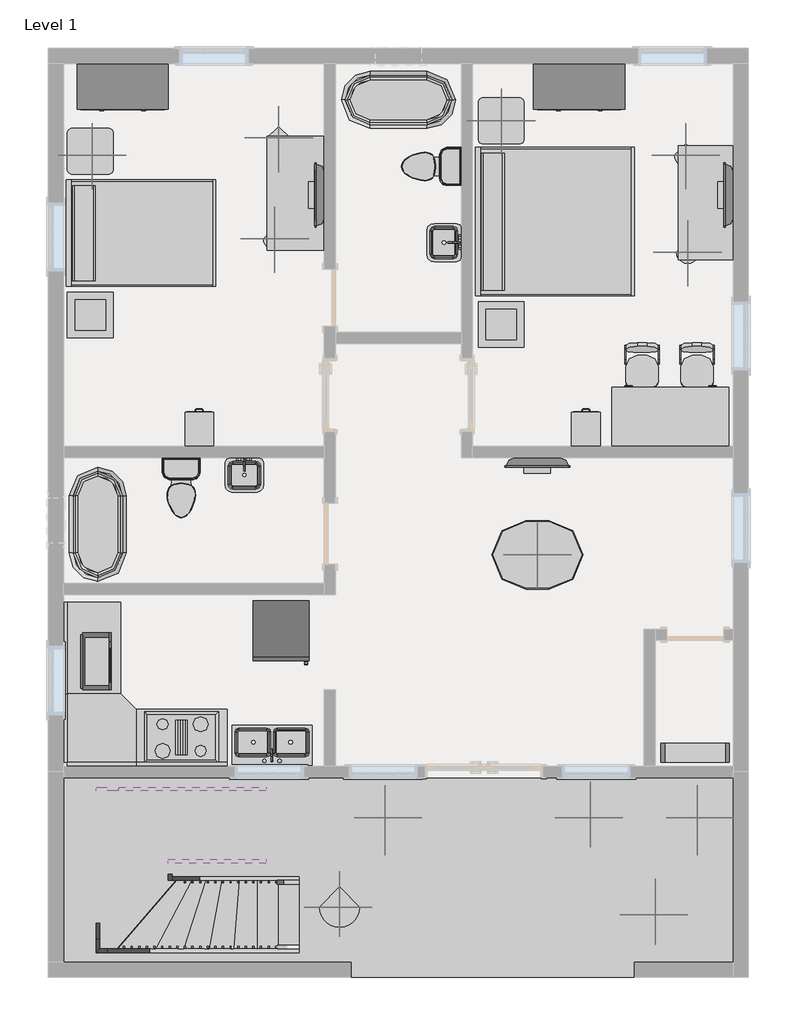
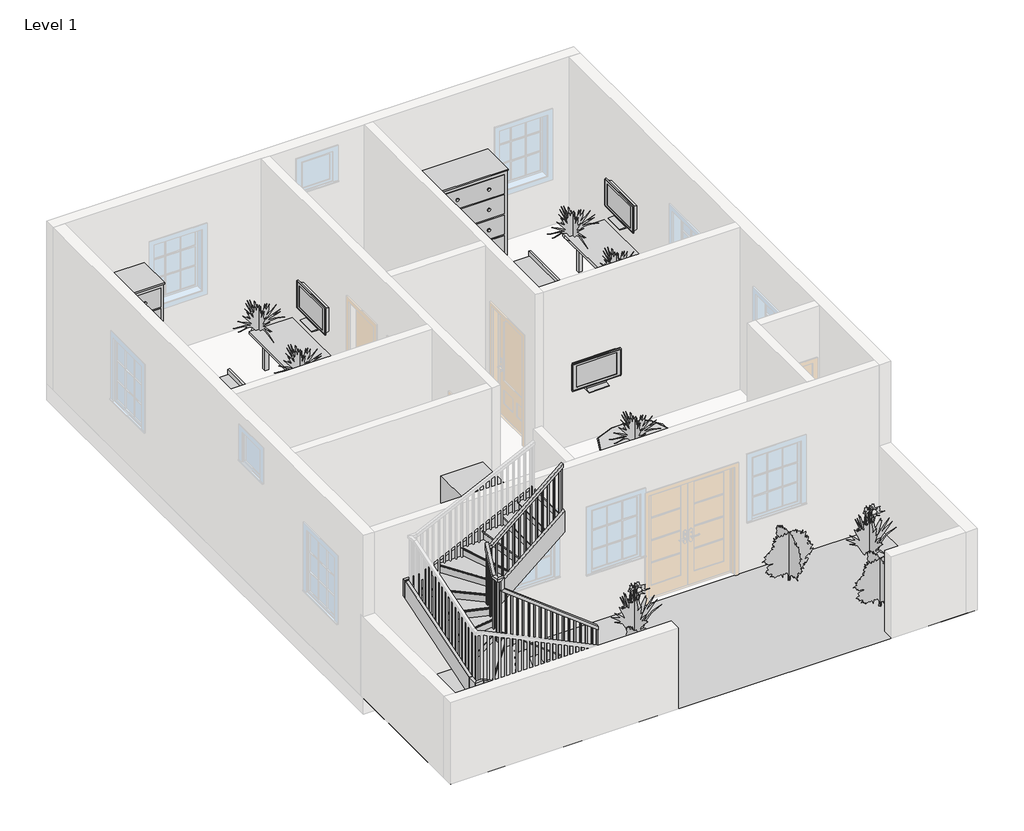
# One storey, part 3 of 3: 21 furniture elements, 12 geographic elements, 9 flow terminals, 9 members, 4 proxies, 1 railing, 1 stair flight.
"""IFC4 building model written with IfcOpenShell, lengths in millimetres."""

from ifc_helpers import new_model, si_unit, frame, origin, place, context, project, spatial, polyline, outline, extrude, faceted_brep, triangles, transform, mapped, element, save
from components import proxy_bb1e6e30, proxy_8a8d5ab2, proxy_a13a33b2, flow_terminal_accce45a, flow_terminal_a53be723, flow_terminal_62a433f7, toilet_domestic_3d_toilet_domestic_3d_f7549cf7, toilet_domestic_3d_toilet_domestic_3d_183bbd19, flow_terminal_b374fae2, furniture_096e7f55, furniture_29cd36cd, furniture_bb55ed6b, furniture_072f6425, furniture_9fa109b2, furniture_3d1d9cbc, furniture_417d203a, furniture_56245f3a, furniture_b5c51a22, furniture_be1c6672, furniture_31d08a24, furniture_2bbcfec9, furniture_65bc2ab2, rpc_plant_tropical_55f6ff97, rpc_plant_tropical_agave_1_5_93a2a214, rpc_plant_tropical_jungle_flame_3_9c4808c2, stair_flight_79a896a8

model = new_model("IFC4")

# Units and contexts
model_context = context("Model", 3, world=origin())
ifc_project = project(units=[si_unit("LENGTHUNIT", "METRE", prefix="MILLI")], contexts=[model_context])

# Site, building, storey
site = spatial("IfcSite", under=ifc_project)
building = spatial("IfcBuilding", under=site)
storey = spatial("IfcBuildingStorey", under=building, Name="Level 1", Elevation=0.0)

# Proxies
placement = place(None, origin())
element("IfcBuildingElementProxy", 1, Name="Building Element Proxy", at=placement, inside=storey, context=model_context, shape_type="Tessellation", body=[
    triangles([(-11433.0067932, 4494.1175446, 0.0), (-2085.8072777, 4494.1175446, 0.0), (-2085.8072777, 1827.1175446, 0.0), (-11433.0067932, 1827.1175446, 0.0)], [[1, 4, 2], [3, 2, 4]], closed=False),
])
proxy_shape = proxy_bb1e6e30(model_context)
element("IfcBuildingElementProxy", 2, Name="Cook Top-4 Unit : 36\" x 20\"", ObjectType="Cook Top-4 Unit : 36\" x 20\"", at=placement, inside=storey, context=model_context, shape_type="MappedRepresentation", body=[
    mapped(proxy_shape, transform((-9655.0073372, 5027.5174997, 0.0), x_axis=(1.0, 0.0, 0.0), y_axis=(0.0, 1.0, 0.0), z_axis=(0.0, 0.0, 1.0))),
])
proxy_2_shape = proxy_8a8d5ab2(model_context)
element("IfcBuildingElementProxy", 3, Name="Microwave : 30\" x 16\" x 18\"", ObjectType="Microwave : 30\" x 16\" x 18\"", at=placement, inside=storey, context=model_context, shape_type="MappedRepresentation", body=[
    mapped(proxy_2_shape, transform((-11151.0878431, 5543.2246223, 0.0), x_axis=(0.0, 1.0000000000000009, 0.0), y_axis=(-1.0000000000000009, 0.0, 0.0), z_axis=(0.0, 0.0, 1.0))),
])
proxy_3_shape = proxy_a13a33b2(model_context)
element("IfcBuildingElementProxy", 4, Name="Refrigerator : 30\" x 32\" RH", ObjectType="Refrigerator : 30\" x 32\" RH", at=placement, inside=storey, context=model_context, shape_type="MappedRepresentation", body=[
    mapped(proxy_3_shape, transform((-8326.2698372, 6467.7685282, 0.0), x_axis=(1.0, 0.0, 0.0), y_axis=(0.0, 1.0, 0.0), z_axis=(0.0, 0.0, 1.0))),
])

# Flow terminals
flow_terminal_shape = flow_terminal_accce45a(model_context)
element("IfcFlowTerminal", 5, ObjectType="Floor Drain - Round : 5\" Strainer - 2\" Drain", at=placement, inside=storey, context=model_context, shape_type="MappedRepresentation", body=[
    mapped(flow_terminal_shape, transform((-7267.4073372, 12215.7174997, 0.0), x_axis=(1.0, 0.0, 0.0), y_axis=(0.0, 1.0, 0.0), z_axis=(0.0, 0.0, 1.0))),
])
element("IfcFlowTerminal", 6, ObjectType="Floor Drain - Round : 5\" Strainer - 2\" Drain", at=placement, inside=storey, context=model_context, shape_type="MappedRepresentation", body=[
    mapped(flow_terminal_shape, transform((-9858.2073372, 7262.7174997, 0.0), x_axis=(1.0, 0.0, 0.0), y_axis=(0.0, 1.0, 0.0), z_axis=(0.0, 0.0, 1.0))),
])
flow_terminal_2_shape = flow_terminal_a53be723(model_context)
element("IfcFlowTerminal", 7, ObjectType="Sink Kitchen-Double : 42\" x 21\"", at=placement, inside=storey, context=model_context, shape_type="MappedRepresentation", body=[
    mapped(flow_terminal_2_shape, transform((-8432.8180967, 4928.2629008, 0.0), x_axis=(-0.9999999999999998, 0.0, 0.0), y_axis=(0.0, -0.9999999999999998, 0.0), z_axis=(0.0, 0.0, 1.0))),
])
flow_terminal_3_shape = flow_terminal_62a433f7(model_context)
element("IfcFlowTerminal", 8, ObjectType="Sink Vanity-Square : 20\" x 18\"", at=placement, inside=storey, context=model_context, shape_type="MappedRepresentation", body=[
    mapped(flow_terminal_3_shape, transform((-6101.3527384, 11647.2067402, 0.0), x_axis=(0.0, -1.0000000000000004, 0.0), y_axis=(1.0000000000000004, 0.0, 0.0), z_axis=(0.0, 0.0, 1.0))),
])
element("IfcFlowTerminal", 9, ObjectType="Sink Vanity-Square : 20\" x 18\"", at=placement, inside=storey, context=model_context, shape_type="MappedRepresentation", body=[
    mapped(flow_terminal_3_shape, transform((-8832.4965778, 8581.1720986, 0.0), x_axis=(1.0, 0.0, 0.0), y_axis=(0.0, 1.0, 0.0), z_axis=(0.0, 0.0, 1.0))),
])
toilet_domestic_3d_toilet_domestic_3d_shape = toilet_domestic_3d_toilet_domestic_3d_f7549cf7(model_context)
toilet_domestic_3d_toilet_domestic_3d_2_shape = toilet_domestic_3d_toilet_domestic_3d_183bbd19(model_context)
element("IfcFlowTerminal", 10, ObjectType="Toilet-Domestic-3D : Toilet-Domestic-3D", at=placement, inside=storey, context=model_context, shape_type="MappedRepresentation", body=[
    mapped(toilet_domestic_3d_toilet_domestic_3d_shape, transform((-6415.9033646, 12647.5174997, 0.0), x_axis=(0.0, -1.0000000000000004, 0.0), y_axis=(1.0000000000000004, 0.0, 0.0), z_axis=(0.0, 0.0, 1.0))),
    mapped(toilet_domestic_3d_toilet_domestic_3d_2_shape, transform((-6415.9033646, 12647.5174997, 0.0), x_axis=(0.0, -1.0000000000000004, 0.0), y_axis=(1.0000000000000004, 0.0, 0.0), z_axis=(0.0, 0.0, 1.0))),
])
element("IfcFlowTerminal", 11, ObjectType="Toilet-Domestic-3D : Toilet-Domestic-3D", at=placement, inside=storey, context=model_context, shape_type="MappedRepresentation", body=[
    mapped(toilet_domestic_3d_toilet_domestic_3d_shape, transform((-9659.4446246, 8266.6214723, 0.0), x_axis=(1.0, 0.0, 0.0), y_axis=(0.0, 1.0, 0.0), z_axis=(0.0, 0.0, 1.0))),
    mapped(toilet_domestic_3d_toilet_domestic_3d_2_shape, transform((-9659.4446246, 8266.6214723, 0.0), x_axis=(1.0, 0.0, 0.0), y_axis=(0.0, 1.0, 0.0), z_axis=(0.0, 0.0, 1.0))),
])
flow_terminal_4_shape = flow_terminal_b374fae2(model_context)
element("IfcFlowTerminal", 12, ObjectType="Tub-Free Standing-3D : 30\" x 60\"", at=placement, inside=storey, context=model_context, shape_type="MappedRepresentation", body=[
    mapped(flow_terminal_4_shape, transform((-6759.4073372, 13536.5174997, 0.0), x_axis=(0.0, 1.0000000000000002, 0.0), y_axis=(-1.0000000000000002, 0.0, 0.0), z_axis=(0.0, 0.0, 1.0))),
])
element("IfcFlowTerminal", 13, ObjectType="Tub-Free Standing-3D : 30\" x 60\"", at=placement, inside=storey, context=model_context, shape_type="MappedRepresentation", body=[
    mapped(flow_terminal_4_shape, transform((-10772.6073372, 7872.3174997, 0.0), x_axis=(1.0, 0.0, 0.0), y_axis=(0.0, 1.0, 0.0), z_axis=(0.0, 0.0, 1.0))),
])

# Furniture
furniture_shape = furniture_096e7f55(model_context)
element("IfcFurniture", 14, ObjectType="Bed-Shaker : Double 56\" x 78\"", at=placement, inside=storey, context=model_context, shape_type="MappedRepresentation", body=[
    mapped(furniture_shape, transform((-11179.0073372, 11777.5674997, 0.0), x_axis=(0.0, 1.0, 0.0), y_axis=(-1.0, 0.0, 0.0), z_axis=(0.0, 0.0, 1.0))),
])
furniture_2_shape = furniture_29cd36cd(model_context)
element("IfcFurniture", 15, ObjectType="Bed-Shaker : King 78\" x 83\"", at=placement, inside=storey, context=model_context, shape_type="MappedRepresentation", body=[
    mapped(furniture_2_shape, transform((-5718.0073372, 11929.9674997, 0.0), x_axis=(0.0, 1.0, 0.0), y_axis=(-1.0, 0.0, 0.0), z_axis=(0.0, 0.0, 1.0))),
])
furniture_3_shape = furniture_bb55ed6b(model_context)
element("IfcFurniture", 16, ObjectType="Cabinet-File 2 Drawer : 15\" x 18\"", at=placement, inside=storey, context=model_context, shape_type="MappedRepresentation", body=[
    mapped(furniture_3_shape, transform((-9548.3766847, 9000.1831995, 0.0), x_axis=(-1.0000000000000004, 0.0, 0.0), y_axis=(0.0, -1.0000000000000004, 0.0), z_axis=(0.0, 0.0, 1.0))),
])
element("IfcFurniture", 17, ObjectType="Cabinet-File 2 Drawer : 15\" x 18\"", at=placement, inside=storey, context=model_context, shape_type="MappedRepresentation", body=[
    mapped(furniture_3_shape, transform((-4385.4037843, 9000.1831995, 0.0), x_axis=(-0.9999999999999998, 0.0, 0.0), y_axis=(0.0, -0.9999999999999998, 0.0), z_axis=(0.0, 0.0, 1.0))),
])
furniture_4_shape = furniture_072f6425(model_context)
element("IfcFurniture", 18, ObjectType="Desk : 60\" x 30\"", at=placement, inside=storey, context=model_context, shape_type="MappedRepresentation", body=[
    mapped(furniture_4_shape, transform((-3889.2073372, 8923.2424997, 0.0), x_axis=(1.0, 0.0, 0.0), y_axis=(0.0, 1.0, 0.0), z_axis=(0.0, 0.0, 1.0))),
])
furniture_5_shape = furniture_9fa109b2(model_context)
element("IfcFurniture", 19, ObjectType="Dresser : 48\" x 72\" x 24\"", at=placement, inside=storey, context=model_context, shape_type="MappedRepresentation", body=[
    mapped(furniture_5_shape, transform((-10173.2140774, 14077.4804538, 0.0), x_axis=(1.0, 0.0, 0.0), y_axis=(0.0, 1.0, 0.0), z_axis=(0.0, 0.0, 1.0))),
])
element("IfcFurniture", 20, ObjectType="Dresser : 48\" x 72\" x 24\"", at=placement, inside=storey, context=model_context, shape_type="MappedRepresentation", body=[
    mapped(furniture_5_shape, transform((-4077.2140774, 14077.4804538, 0.0), x_axis=(1.0, 0.0, 0.0), y_axis=(0.0, 1.0, 0.0), z_axis=(0.0, 0.0, 1.0))),
])
furniture_6_shape = furniture_3d1d9cbc(model_context)
element("IfcFurniture", 21, ObjectType="Seating-Auditorium : 18\" x 24\" x 30\"", at=placement, inside=storey, context=model_context, shape_type="MappedRepresentation", body=[
    mapped(furniture_6_shape, transform((-3347.4794684, 10195.7929095, 0.0), x_axis=(-1.0000000000000004, 0.0, 0.0), y_axis=(0.0, -1.0000000000000004, 0.0), z_axis=(0.0, 0.0, 1.0))),
])
element("IfcFurniture", 22, ObjectType="Seating-Auditorium : 18\" x 24\" x 30\"", at=placement, inside=storey, context=model_context, shape_type="MappedRepresentation", body=[
    mapped(furniture_6_shape, transform((-2610.8794684, 10195.7929095, 0.0), x_axis=(-1.0, 0.0, 0.0), y_axis=(0.0, -1.0, 0.0), z_axis=(0.0, 0.0, 1.0))),
])
furniture_7_shape = furniture_417d203a(model_context)
element("IfcFurniture", 23, ObjectType="Shelving : 36\" x 10\" x 72\"", at=placement, inside=storey, context=model_context, shape_type="MappedRepresentation", body=[
    mapped(furniture_7_shape, transform((-2797.0073372, 5129.1174997, 0.0), x_axis=(1.0, 0.0, 0.0), y_axis=(0.0, 1.0, 0.0), z_axis=(0.0, 0.0, 1.0))),
])
furniture_8_shape = furniture_56245f3a(model_context)
element("IfcFurniture", 24, ObjectType="TV - Flat Screen : 32\"", at=placement, inside=storey, context=model_context, shape_type="MappedRepresentation", body=[
    mapped(furniture_8_shape, transform((-7808.5459609, 12262.5729855, 1041.4), x_axis=(0.0, -1.0000000000000004, 0.0), y_axis=(1.0000000000000004, 0.0, 0.0), z_axis=(0.0, 0.0, 1.0))),
])
element("IfcFurniture", 25, ObjectType="TV - Flat Screen : 32\"", at=placement, inside=storey, context=model_context, shape_type="MappedRepresentation", body=[
    mapped(furniture_8_shape, transform((-2347.5459609, 12262.5729855, 1041.4), x_axis=(0.0, -1.0000000000000004, 0.0), y_axis=(1.0000000000000004, 0.0, 0.0), z_axis=(0.0, 0.0, 1.0))),
])
element("IfcFurniture", 26, ObjectType="TV - Flat Screen : 32\"", at=placement, inside=storey, context=model_context, shape_type="MappedRepresentation", body=[
    mapped(furniture_8_shape, transform((-4901.2628231, 8702.778876, 1041.4), x_axis=(1.0, 0.0, 0.0), y_axis=(0.0, 1.0, 0.0), z_axis=(0.0, 0.0, 1.0))),
])
furniture_9_shape = furniture_b5c51a22(model_context)
element("IfcFurniture", 27, ObjectType="Table-Coffee : 24\" x 24\" x 24\"", at=placement, inside=storey, context=model_context, shape_type="MappedRepresentation", body=[
    mapped(furniture_9_shape, transform((-10892.4731039, 10571.1064219, 0.0), x_axis=(1.0, 0.0, 0.0), y_axis=(0.0, 1.0, 0.0), z_axis=(0.0, 0.0, 1.0))),
])
element("IfcFurniture", 28, ObjectType="Table-Coffee : 24\" x 24\" x 24\"", at=placement, inside=storey, context=model_context, shape_type="MappedRepresentation", body=[
    mapped(furniture_9_shape, transform((-5406.0731039, 10444.1064219, 0.0), x_axis=(1.0, 0.0, 0.0), y_axis=(0.0, 1.0, 0.0), z_axis=(0.0, 0.0, 1.0))),
])
furniture_10_shape = furniture_be1c6672(model_context)
element("IfcFurniture", 29, ObjectType="Table-Dining Oval : 36\" x 48\"", at=placement, inside=storey, context=model_context, shape_type="MappedRepresentation", body=[
    mapped(furniture_10_shape, transform((-4503.3876651, 7824.0158603, 0.0), x_axis=(1.0, 0.0, 0.0), y_axis=(0.0, 1.0, 0.0), z_axis=(0.0, 0.0, 1.0))),
])
furniture_11_shape = furniture_31d08a24(model_context)
element("IfcFurniture", 30, ObjectType="Table-End : 24\" x 24\"", at=placement, inside=storey, context=model_context, shape_type="MappedRepresentation", body=[
    mapped(furniture_11_shape, transform((-11182.7409675, 12698.3174997, 0.0), x_axis=(1.0, 0.0, 0.0), y_axis=(0.0, 1.0, 0.0), z_axis=(0.0, 0.0, 1.0))),
])
element("IfcFurniture", 31, ObjectType="Table-End : 24\" x 24\"", at=placement, inside=storey, context=model_context, shape_type="MappedRepresentation", body=[
    mapped(furniture_11_shape, transform((-5696.3409675, 13104.7174997, 0.0), x_axis=(1.0, 0.0, 0.0), y_axis=(0.0, 1.0, 0.0), z_axis=(0.0, 0.0, 1.0))),
])
furniture_12_shape = furniture_2bbcfec9(model_context)
element("IfcFurniture", 32, ObjectType="Table-Rectangular : 72\" x 30\"", at=placement, inside=storey, context=model_context, shape_type="MappedRepresentation", body=[
    mapped(furniture_12_shape, transform((-8131.0073372, 12291.9174997, 0.0), x_axis=(0.0, 1.0000000000000002, 0.0), y_axis=(-1.0000000000000002, 0.0, 0.0), z_axis=(0.0, 0.0, 1.0))),
])
element("IfcFurniture", 33, ObjectType="Table-Rectangular : 72\" x 30\"", at=placement, inside=storey, context=model_context, shape_type="MappedRepresentation", body=[
    mapped(furniture_12_shape, transform((-2644.6073372, 12164.9174997, 0.0), x_axis=(0.0, 1.0000000000000002, 0.0), y_axis=(-1.0000000000000002, 0.0, 0.0), z_axis=(0.0, 0.0, 1.0))),
])
furniture_13_shape = furniture_65bc2ab2(model_context)
element("IfcFurniture", 34, ObjectType="Work Station Cubicle : 96\" x 96\"", at=placement, inside=storey, context=model_context, shape_type="MappedRepresentation", body=[
    mapped(furniture_13_shape, transform((-11724.8303449, 4778.2492519, 0.0), x_axis=(0.0, 1.0000000000000002, 0.0), y_axis=(-1.0000000000000002, 0.0, 0.0), z_axis=(0.0, 0.0, 1.0))),
])

# Geographic elements
rpc_plant_tropical_shape = rpc_plant_tropical_55f6ff97(model_context)
element("IfcGeographicElement", 35, ObjectType="RPC Plant - Tropical", at=placement, inside=storey, context=model_context, shape_type="MappedRepresentation", body=[
    mapped(rpc_plant_tropical_shape, transform((-2771.6073372, 3960.7174997, 0.0), x_axis=(1.0, 0.0, 0.0), y_axis=(0.0, 1.0, 0.0), z_axis=(0.0, 0.0, 1.0))),
])
element("IfcGeographicElement", 36, ObjectType="RPC Plant - Tropical", at=placement, inside=storey, context=model_context, shape_type="MappedRepresentation", body=[
    mapped(rpc_plant_tropical_shape, transform((-6937.2073372, 3960.7174997, 0.0), x_axis=(1.0, 0.0, 0.0), y_axis=(0.0, 1.0, 0.0), z_axis=(0.0, 0.0, 1.0))),
])
rpc_plant_tropical_agave_1_5_shape = rpc_plant_tropical_agave_1_5_93a2a214(model_context)
element("IfcGeographicElement", 37, ObjectType="RPC Plant - Tropical : Agave - 1.5'", at=placement, inside=storey, context=model_context, shape_type="MappedRepresentation", body=[
    mapped(rpc_plant_tropical_agave_1_5_shape, transform((-10848.8073372, 12799.9174997, 609.6), x_axis=(1.0, 0.0, 0.0), y_axis=(0.0, 1.0, 0.0), z_axis=(0.0, 0.0, 1.0))),
])
element("IfcGeographicElement", 38, ObjectType="RPC Plant - Tropical : Agave - 1.5'", at=placement, inside=storey, context=model_context, shape_type="MappedRepresentation", body=[
    mapped(rpc_plant_tropical_agave_1_5_shape, transform((-8359.6073372, 13028.5174997, 660.4), x_axis=(1.0, 0.0, 0.0), y_axis=(0.0, 1.0, 0.0), z_axis=(0.0, 0.0, 1.0))),
])
element("IfcGeographicElement", 39, ObjectType="RPC Plant - Tropical : Agave - 1.5'", at=placement, inside=storey, context=model_context, shape_type="MappedRepresentation", body=[
    mapped(rpc_plant_tropical_agave_1_5_shape, transform((-8410.4073372, 11682.3174997, 660.4), x_axis=(1.0, 0.0, 0.0), y_axis=(0.0, 1.0, 0.0), z_axis=(0.0, 0.0, 1.0))),
])
element("IfcGeographicElement", 40, ObjectType="RPC Plant - Tropical : Agave - 1.5'", at=placement, inside=storey, context=model_context, shape_type="MappedRepresentation", body=[
    mapped(rpc_plant_tropical_agave_1_5_shape, transform((-5387.8073372, 13257.1174997, 609.6), x_axis=(1.0, 0.0, 0.0), y_axis=(0.0, 1.0, 0.0), z_axis=(0.0, 0.0, 1.0))),
])
element("IfcGeographicElement", 41, ObjectType="RPC Plant - Tropical : Agave - 1.5'", at=placement, inside=storey, context=model_context, shape_type="MappedRepresentation", body=[
    mapped(rpc_plant_tropical_agave_1_5_shape, transform((-2924.0073372, 12799.9174997, 660.4), x_axis=(1.0, 0.0, 0.0), y_axis=(0.0, 1.0, 0.0), z_axis=(0.0, 0.0, 1.0))),
])
element("IfcGeographicElement", 42, ObjectType="RPC Plant - Tropical : Agave - 1.5'", at=placement, inside=storey, context=model_context, shape_type="MappedRepresentation", body=[
    mapped(rpc_plant_tropical_agave_1_5_shape, transform((-2898.6073372, 11504.5174997, 660.4), x_axis=(1.0, 0.0, 0.0), y_axis=(0.0, 1.0, 0.0), z_axis=(0.0, 0.0, 1.0))),
])
element("IfcGeographicElement", 43, ObjectType="RPC Plant - Tropical : Agave - 1.5'", at=placement, inside=storey, context=model_context, shape_type="MappedRepresentation", body=[
    mapped(rpc_plant_tropical_agave_1_5_shape, transform((-4905.2073372, 7465.9174997, 736.6), x_axis=(1.0, 0.0, 0.0), y_axis=(0.0, 1.0, 0.0), z_axis=(0.0, 0.0, 1.0))),
])
rpc_plant_tropical_jungle_flame_3_shape = rpc_plant_tropical_jungle_flame_3_9c4808c2(model_context)
element("IfcGeographicElement", 44, ObjectType="RPC Plant - Tropical : Jungle Flame - 3'", at=placement, inside=storey, context=model_context, shape_type="MappedRepresentation", body=[
    mapped(rpc_plant_tropical_jungle_flame_3_shape, transform((-3330.4073372, 2665.3174997, 0.0), x_axis=(1.0, 0.0, 0.0), y_axis=(0.0, 1.0, 0.0), z_axis=(0.0, 0.0, 1.0))),
])
element("IfcGeographicElement", 45, ObjectType="RPC Plant - Tropical : Jungle Flame - 3'", at=placement, inside=storey, context=model_context, shape_type="MappedRepresentation", body=[
    mapped(rpc_plant_tropical_jungle_flame_3_shape, transform((-4194.0073372, 3960.7174997, 0.0), x_axis=(1.0, 0.0, 0.0), y_axis=(0.0, 1.0, 0.0), z_axis=(0.0, 0.0, 1.0))),
])
element("IfcGeographicElement", 46, ObjectType="RPC Plant - Tropical : Jungle Flame - 3'", at=placement, inside=storey, context=model_context, shape_type="MappedRepresentation", body=[
    mapped(rpc_plant_tropical_jungle_flame_3_shape, transform((-7546.8073372, 2766.9174997, 0.0), x_axis=(1.0, 0.0, 0.0), y_axis=(0.0, 1.0, 0.0), z_axis=(0.0, 0.0, 1.0))),
])

# Members
element("IfcMember", 47, ObjectType="Stringer - 2\" Width", at=placement, inside=storey, context=model_context, shape_type="SweptSolid", body=[
    extrude(outline(polyline([(0.0, -8086.227471), (236.3829991, -8086.227471), (1471.7792005, -10648.1727738), (1133.3926217, -10648.1727738), (0.0, -8297.7608978), (0.0, -8086.227471)])), frame((0.0, 2157.3174997, 0.0), z_axis=(0.0, 1.0, 0.0), x_axis=(0.0, 0.0, 1.0)), (0.0, 0.0, 1.0), 50.8),
])
element("IfcMember", 48, ObjectType="Stringer - 2\" Width", at=placement, inside=storey, context=model_context, shape_type="SweptSolid", body=[
    extrude(outline(polyline([(-10648.1727738, 2208.1174997), (-10648.1727738, 2157.3174997), (-10798.0073372, 2157.3174997), (-10747.2073372, 2208.1174997), (-10648.1727738, 2208.1174997)])), frame((0.0, 0.0, 1133.3926217), z_axis=(0.0, 0.0, 1.0), x_axis=(1.0, 0.0, 0.0)), (0.0, 0.0, 1.0), 338.3865788),
])
element("IfcMember", 49, ObjectType="Stringer - 2\" Width", at=placement, inside=storey, context=model_context, shape_type="SweptSolid", body=[
    extrude(outline(polyline([(-10747.2073372, 2208.1174997), (-10798.0073372, 2157.3174997), (-10798.0073372, 2336.424848), (-10747.2073372, 2336.424848), (-10747.2073372, 2208.1174997)])), frame((0.0, 0.0, 1133.3926217), z_axis=(0.0, 0.0, 1.0), x_axis=(1.0, 0.0, 0.0)), (0.0, 0.0, 1.0), 338.3865788),
])
element("IfcMember", 50, ObjectType="Stringer - 2\" Width", at=placement, inside=storey, context=model_context, shape_type="SweptSolid", body=[
    extrude(outline(polyline([(2336.424848, 1133.3926217), (2336.424848, 1471.7792005), (4286.2118675, 2088.9485372), (4316.3174997, 2088.9485372), (4316.3174997, 1760.0913444), (2336.424848, 1133.3926217)])), frame((-10798.0073372, 0.0, 0.0), z_axis=(1.0, 0.0, 0.0), x_axis=(0.0, 1.0, 0.0)), (0.0, 0.0, 1.0), 50.8),
])
element("IfcMember", 51, ObjectType="Stringer - 2\" Width", at=placement, inside=storey, context=model_context, shape_type="SweptSolid", body=[
    extrude(outline(polyline([(-10798.0073372, 4316.3174997), (-10798.0073372, 4367.1174997), (-10498.063024, 4367.1174997), (-10498.063024, 4316.3174997), (-10798.0073372, 4316.3174997)])), frame((0.0, 0.0, 1769.2436593), z_axis=(0.0, 0.0, 1.0), x_axis=(1.0, 0.0, 0.0)), (0.0, 0.0, 1.0), 319.7048779),
])
element("IfcMember", 52, ObjectType="Stringer - 2\" Width", at=placement, inside=storey, context=model_context, shape_type="SweptSolid", body=[
    extrude(outline(polyline([(0.0, -8086.227471), (183.6172577, -8086.227471), (1488.0817916, -9782.0073372), (1103.5342512, -9782.0073372), (0.0, -8347.4331375), (0.0, -8086.227471)])), frame((0.0, 3122.5174997, 0.0), z_axis=(0.0, 1.0, 0.0), x_axis=(0.0, 0.0, 1.0)), (0.0, 0.0, 1.0), 50.8),
])
element("IfcMember", 53, ObjectType="Stringer - 2\" Width", at=placement, inside=storey, context=model_context, shape_type="SweptSolid", body=[
    extrude(outline(polyline([(3122.5174997, 1142.6117279), (3122.5174997, 1735.04182), (3283.2970754, 2070.7015224), (3351.1174997, 2070.7015224), (3351.1174997, 1506.7262904), (3176.7081665, 1142.6117279), (3122.5174997, 1142.6117279)])), frame((-9832.8073372, 0.0, 0.0), z_axis=(1.0, 0.0, 0.0), x_axis=(0.0, 1.0, 0.0)), (0.0, 0.0, 1.0), 50.8),
])
element("IfcMember", 54, ObjectType="Stringer - 2\" Width", at=placement, inside=storey, context=model_context, shape_type="SweptSolid", body=[
    extrude(outline(polyline([(2070.7015224, -9832.8073372), (1670.0735122, -9832.8073372), (2786.3187936, -8524.2221093), (3186.9468038, -8524.2221093), (2070.7015224, -9832.8073372)])), frame((0.0, 3351.1174997, 0.0), z_axis=(0.0, 1.0, 0.0), x_axis=(0.0, 0.0, 1.0)), (0.0, 0.0, 1.0), 50.8),
])
element("IfcMember", 55, ObjectType="Stringer - 2\" Width", at=placement, inside=storey, context=model_context, shape_type="SweptSolid", body=[
    extrude(outline(polyline([(2088.9485372, -10498.063024), (1769.2436593, -10498.063024), (2715.8753355, -8524.2221093), (3035.5802134, -8524.2221093), (2088.9485372, -10498.063024)])), frame((0.0, 4316.3174997, 0.0), z_axis=(0.0, 1.0, 0.0), x_axis=(0.0, 0.0, 1.0)), (0.0, 0.0, 1.0), 50.8),
])

# Railing
element("IfcRailing", 56, ObjectType="Handrail - Rectangular", at=placement, inside=storey, context=model_context, shape_type="SolidModel", body=[
    faceted_brep([(-8086.227471, 3071.7174997, 1038.1405445), (-8086.227471, 3071.7174997, 974.0492877), (-8086.227471, 3122.5174997, 974.0492877), (-8086.227471, 3122.5174997, 1038.1405445), (-9756.6073372, 3071.7174997, 2323.06634), (-9807.4073372, 3071.7174997, 2298.05256), (-9807.4073372, 3122.5174997, 2298.05256), (-9756.6073372, 3122.5174997, 2323.06634), (-9756.6073372, 3071.7174997, 2536.3709838), (-9807.4073372, 3071.7174997, 2485.5709838), (-9807.4073372, 3122.5174997, 2485.5709838), (-9756.6073372, 3122.5174997, 2536.3709838), (-9883.6073372, 3071.7174997, 2536.3709838), (-9883.6073372, 3071.7174997, 2485.5709838), (-9832.8073372, 3122.5174997, 2485.5709838), (-9832.8073372, 3122.5174997, 2536.3709838), (-9883.6073372, 3198.7174997, 2536.3709838), (-9883.6073372, 3230.7115434, 2485.5709838), (-9832.8073372, 3230.7115434, 2485.5709838), (-9832.8073372, 3198.7174997, 2536.3709838), (-9883.6073372, 3427.3174997, 3013.6194629), (-9832.8073372, 3427.3174997, 3013.6194629), (-9832.8073372, 3427.3174997, 2896.0254615), (-9883.6073372, 3427.3174997, 2896.0254615)], [[[0, 1, 2, 3]], [[1, 0, 4, 5]], [[2, 1, 5, 6]], [[3, 2, 6, 7]], [[0, 3, 7, 4]], [[5, 4, 8, 9]], [[6, 5, 9, 10]], [[7, 6, 10, 11]], [[4, 7, 11, 8]], [[9, 8, 12, 13]], [[10, 9, 13, 14]], [[11, 10, 14, 15]], [[8, 11, 15, 12]], [[13, 12, 16, 17]], [[14, 13, 17, 18]], [[15, 14, 18, 19]], [[12, 15, 19, 16]], [[20, 21, 22, 23]], [[17, 16, 20, 23]], [[18, 17, 23, 22]], [[19, 18, 22, 21]], [[16, 19, 21, 20]]]),
    faceted_brep([(-9858.2073372, 3452.7174997, 2953.5535672), (-9858.2073372, 3452.7174997, 2902.7535672), (-9858.2073372, 3401.9174997, 2902.7535672), (-9858.2073372, 3401.9174997, 2953.5535672), (-9787.791502, 3452.7174997, 2953.5535672), (-9769.0681502, 3452.7174997, 2902.7535672), (-9769.0681502, 3401.9174997, 2902.7535672), (-9787.791502, 3401.9174997, 2953.5535672), (-8524.2221093, 3452.7174997, 4031.3995815), (-8524.2221093, 3401.9174997, 4031.3995815), (-8524.2221093, 3401.9174997, 3964.6282464), (-8524.2221093, 3452.7174997, 3964.6282464)], [[[0, 1, 2, 3]], [[1, 0, 4, 5]], [[2, 1, 5, 6]], [[3, 2, 6, 7]], [[0, 3, 7, 4]], [[8, 9, 10, 11]], [[5, 4, 8, 11]], [[6, 5, 11, 10]], [[7, 6, 10, 9]], [[4, 7, 9, 8]]]),
    extrude(outline(polyline([(3934.9053915, -8559.066502), (3918.65542, -8578.116502), (2878.6666667, -8578.116502), (2878.6666667, -8559.066502), (3934.9053915, -8559.066502)])), frame((0.0, 3417.7924997, 0.0), z_axis=(0.0, 1.0, 0.0), x_axis=(0.0, 0.0, 1.0)), (0.0, 0.0, 1.0), 19.05),
    extrude(outline(polyline([(3848.238877, -8660.666502), (3831.9889056, -8679.716502), (2878.6666667, -8679.716502), (2878.6666667, -8660.666502), (3848.238877, -8660.666502)])), frame((0.0, 3417.7924997, 0.0), z_axis=(0.0, 1.0, 0.0), x_axis=(0.0, 0.0, 1.0)), (0.0, 0.0, 1.0), 19.05),
    extrude(outline(polyline([(3761.5723626, -8762.266502), (3745.3223911, -8781.316502), (2878.6666667, -8781.316502), (2878.6666667, -8762.266502), (3761.5723626, -8762.266502)])), frame((0.0, 3417.7924997, 0.0), z_axis=(0.0, 1.0, 0.0), x_axis=(0.0, 0.0, 1.0)), (0.0, 0.0, 1.0), 19.05),
    extrude(outline(polyline([(3674.9058481, -8863.866502), (3658.6558766, -8882.916502), (2709.3333333, -8882.916502), (2709.3333333, -8863.866502), (3674.9058481, -8863.866502)])), frame((0.0, 3417.7924997, 0.0), z_axis=(0.0, 1.0, 0.0), x_axis=(0.0, 0.0, 1.0)), (0.0, 0.0, 1.0), 19.05),
    extrude(outline(polyline([(3588.2393336, -8965.466502), (3571.9893622, -8984.516502), (2709.3333333, -8984.516502), (2709.3333333, -8965.466502), (3588.2393336, -8965.466502)])), frame((0.0, 3417.7924997, 0.0), z_axis=(0.0, 1.0, 0.0), x_axis=(0.0, 0.0, 1.0)), (0.0, 0.0, 1.0), 19.05),
    extrude(outline(polyline([(3501.5728192, -9067.066502), (3485.3228477, -9086.116502), (2709.3333333, -9086.116502), (2709.3333333, -9067.066502), (3501.5728192, -9067.066502)])), frame((0.0, 3417.7924997, 0.0), z_axis=(0.0, 1.0, 0.0), x_axis=(0.0, 0.0, 1.0)), (0.0, 0.0, 1.0), 19.05),
    extrude(outline(polyline([(3414.9063047, -9168.666502), (3398.6563332, -9187.716502), (2540.0, -9187.716502), (2540.0, -9168.666502), (3414.9063047, -9168.666502)])), frame((0.0, 3417.7924997, 0.0), z_axis=(0.0, 1.0, 0.0), x_axis=(0.0, 0.0, 1.0)), (0.0, 0.0, 1.0), 19.05),
    extrude(outline(polyline([(3328.2397902, -9270.266502), (3311.9898188, -9289.316502), (2540.0, -9289.316502), (2540.0, -9270.266502), (3328.2397902, -9270.266502)])), frame((0.0, 3417.7924997, 0.0), z_axis=(0.0, 1.0, 0.0), x_axis=(0.0, 0.0, 1.0)), (0.0, 0.0, 1.0), 19.05),
    extrude(outline(polyline([(3241.5732758, -9371.866502), (3225.3233043, -9390.916502), (2370.6666667, -9390.916502), (2370.6666667, -9371.866502), (3241.5732758, -9371.866502)])), frame((0.0, 3417.7924997, 0.0), z_axis=(0.0, 1.0, 0.0), x_axis=(0.0, 0.0, 1.0)), (0.0, 0.0, 1.0), 19.05),
    extrude(outline(polyline([(3154.9067613, -9473.466502), (3138.6567898, -9492.516502), (2370.6666667, -9492.516502), (2370.6666667, -9473.466502), (3154.9067613, -9473.466502)])), frame((0.0, 3417.7924997, 0.0), z_axis=(0.0, 1.0, 0.0), x_axis=(0.0, 0.0, 1.0)), (0.0, 0.0, 1.0), 19.05),
    extrude(outline(polyline([(3068.2402468, -9575.066502), (3051.9902754, -9594.116502), (2201.3333333, -9594.116502), (2201.3333333, -9575.066502), (3068.2402468, -9575.066502)])), frame((0.0, 3417.7924997, 0.0), z_axis=(0.0, 1.0, 0.0), x_axis=(0.0, 0.0, 1.0)), (0.0, 0.0, 1.0), 19.05),
    extrude(outline(polyline([(2981.5737324, -9676.666502), (2965.3237609, -9695.716502), (2032.0, -9695.716502), (2032.0, -9676.666502), (2981.5737324, -9676.666502)])), frame((0.0, 3417.7924997, 0.0), z_axis=(0.0, 1.0, 0.0), x_axis=(0.0, 0.0, 1.0)), (0.0, 0.0, 1.0), 19.05),
    extrude(outline(polyline([(3309.2244351, 2649.4824367), (3328.2744351, 2689.2531433), (3328.2744351, 1693.3333333), (3309.2244351, 1693.3333333), (3309.2244351, 2649.4824367)])), frame((-9867.7323372, 0.0, 0.0), z_axis=(1.0, 0.0, 0.0), x_axis=(0.0, 1.0, 0.0)), (0.0, 0.0, 1.0), 19.05),
    extrude(outline(polyline([(3207.6244351, 2437.3720015), (3226.6744351, 2477.1427081), (3226.6744351, 1524.0), (3207.6244351, 1524.0), (3207.6244351, 2437.3720015)])), frame((-9867.7323372, 0.0, 0.0), z_axis=(1.0, 0.0, 0.0), x_axis=(0.0, 1.0, 0.0)), (0.0, 0.0, 1.0), 19.05),
    extrude(outline(polyline([(2217.1871214, -9702.302471), (2231.8411752, -9721.352471), (1354.6666667, -9721.352471), (1354.6666667, -9702.302471), (2217.1871214, -9702.302471)])), frame((0.0, 3087.5924997, 0.0), z_axis=(0.0, 1.0, 0.0), x_axis=(0.0, 0.0, 1.0)), (0.0, 0.0, 1.0), 19.05),
    extrude(outline(polyline([(2139.0321679, -9600.702471), (2153.6862217, -9619.752471), (1185.3333333, -9619.752471), (1185.3333333, -9600.702471), (2139.0321679, -9600.702471)])), frame((0.0, 3087.5924997, 0.0), z_axis=(0.0, 1.0, 0.0), x_axis=(0.0, 0.0, 1.0)), (0.0, 0.0, 1.0), 19.05),
    extrude(outline(polyline([(2060.8916103, -9499.102471), (2075.5456641, -9518.152471), (1016.0, -9518.152471), (1016.0, -9499.102471), (2060.8916103, -9499.102471)])), frame((0.0, 3087.5924997, 0.0), z_axis=(0.0, 1.0, 0.0), x_axis=(0.0, 0.0, 1.0)), (0.0, 0.0, 1.0), 19.05),
    extrude(outline(polyline([(1982.7366567, -9397.502471), (1997.3907105, -9416.552471), (1016.0, -9416.552471), (1016.0, -9397.502471), (1982.7366567, -9397.502471)])), frame((0.0, 3087.5924997, 0.0), z_axis=(0.0, 1.0, 0.0), x_axis=(0.0, 0.0, 1.0)), (0.0, 0.0, 1.0), 19.05),
    extrude(outline(polyline([(1904.5817032, -9295.902471), (1919.235757, -9314.952471), (846.6666667, -9314.952471), (846.6666667, -9295.902471), (1904.5817032, -9295.902471)])), frame((0.0, 3087.5924997, 0.0), z_axis=(0.0, 1.0, 0.0), x_axis=(0.0, 0.0, 1.0)), (0.0, 0.0, 1.0), 19.05),
    extrude(outline(polyline([(1826.4267497, -9194.302471), (1841.0808035, -9213.352471), (846.6666667, -9213.352471), (846.6666667, -9194.302471), (1826.4267497, -9194.302471)])), frame((0.0, 3087.5924997, 0.0), z_axis=(0.0, 1.0, 0.0), x_axis=(0.0, 0.0, 1.0)), (0.0, 0.0, 1.0), 19.05),
    extrude(outline(polyline([(1748.2717961, -9092.702471), (1762.9258499, -9111.752471), (677.3333333, -9111.752471), (677.3333333, -9092.702471), (1748.2717961, -9092.702471)])), frame((0.0, 3087.5924997, 0.0), z_axis=(0.0, 1.0, 0.0), x_axis=(0.0, 0.0, 1.0)), (0.0, 0.0, 1.0), 19.05),
    extrude(outline(polyline([(1670.1168426, -8991.102471), (1684.7708964, -9010.152471), (677.3333333, -9010.152471), (677.3333333, -8991.102471), (1670.1168426, -8991.102471)])), frame((0.0, 3087.5924997, 0.0), z_axis=(0.0, 1.0, 0.0), x_axis=(0.0, 0.0, 1.0)), (0.0, 0.0, 1.0), 19.05),
    extrude(outline(polyline([(1591.9618891, -8889.502471), (1606.6159429, -8908.552471), (677.3333333, -8908.552471), (677.3333333, -8889.502471), (1591.9618891, -8889.502471)])), frame((0.0, 3087.5924997, 0.0), z_axis=(0.0, 1.0, 0.0), x_axis=(0.0, 0.0, 1.0)), (0.0, 0.0, 1.0), 19.05),
    extrude(outline(polyline([(1513.8069355, -8787.902471), (1528.4609893, -8806.952471), (508.0, -8806.952471), (508.0, -8787.902471), (1513.8069355, -8787.902471)])), frame((0.0, 3087.5924997, 0.0), z_axis=(0.0, 1.0, 0.0), x_axis=(0.0, 0.0, 1.0)), (0.0, 0.0, 1.0), 19.05),
    extrude(outline(polyline([(1435.651982, -8686.302471), (1450.3060358, -8705.352471), (508.0, -8705.352471), (508.0, -8686.302471), (1435.651982, -8686.302471)])), frame((0.0, 3087.5924997, 0.0), z_axis=(0.0, 1.0, 0.0), x_axis=(0.0, 0.0, 1.0)), (0.0, 0.0, 1.0), 19.05),
    extrude(outline(polyline([(1357.4970285, -8584.702471), (1372.1510823, -8603.752471), (338.6666667, -8603.752471), (338.6666667, -8584.702471), (1357.4970285, -8584.702471)])), frame((0.0, 3087.5924997, 0.0), z_axis=(0.0, 1.0, 0.0), x_axis=(0.0, 0.0, 1.0)), (0.0, 0.0, 1.0), 19.05),
    extrude(outline(polyline([(1279.3420749, -8483.102471), (1293.9961287, -8502.152471), (338.6666667, -8502.152471), (338.6666667, -8483.102471), (1279.3420749, -8483.102471)])), frame((0.0, 3087.5924997, 0.0), z_axis=(0.0, 1.0, 0.0), x_axis=(0.0, 0.0, 1.0)), (0.0, 0.0, 1.0), 19.05),
    extrude(outline(polyline([(1201.1871214, -8381.502471), (1215.8411752, -8400.552471), (338.6666667, -8400.552471), (338.6666667, -8381.502471), (1201.1871214, -8381.502471)])), frame((0.0, 3087.5924997, 0.0), z_axis=(0.0, 1.0, 0.0), x_axis=(0.0, 0.0, 1.0)), (0.0, 0.0, 1.0), 19.05),
    extrude(outline(polyline([(1123.0321679, -8279.902471), (1137.6862217, -8298.952471), (169.3333333, -8298.952471), (169.3333333, -8279.902471), (1123.0321679, -8279.902471)])), frame((0.0, 3087.5924997, 0.0), z_axis=(0.0, 1.0, 0.0), x_axis=(0.0, 0.0, 1.0)), (0.0, 0.0, 1.0), 19.05),
    extrude(outline(polyline([(1044.8772144, -8178.302471), (1059.5312681, -8197.352471), (169.3333333, -8197.352471), (169.3333333, -8178.302471), (1044.8772144, -8178.302471)])), frame((0.0, 3087.5924997, 0.0), z_axis=(0.0, 1.0, 0.0), x_axis=(0.0, 0.0, 1.0)), (0.0, 0.0, 1.0), 19.05),
    extrude(outline(polyline([(-9797.316502, 3417.7924997), (-9797.316502, 3436.8424997), (-9778.266502, 3436.8424997), (-9778.266502, 3417.7924997), (-9797.316502, 3417.7924997)])), frame((0.0, 0.0, 2032.0), z_axis=(0.0, 0.0, 1.0), x_axis=(1.0, 0.0, 0.0)), (0.0, 0.0, 1.0), 870.7535672),
    extrude(outline(polyline([(3417.7924997, 2876.1401082), (3436.8424997, 2915.9108148), (3436.8424997, 1862.6666667), (3417.7924997, 1862.6666667), (3417.7924997, 2876.1401082)])), frame((-9867.7323372, 0.0, 0.0), z_axis=(1.0, 0.0, 0.0), x_axis=(0.0, 1.0, 0.0)), (0.0, 0.0, 1.0), 19.05),
    extrude(outline(polyline([(3389.02119, 2816.0742125), (3408.07119, 2855.844919), (3408.07119, 1862.6666667), (3389.02119, 1862.6666667), (3389.02119, 2816.0742125)])), frame((-9867.7323372, 0.0, 0.0), z_axis=(1.0, 0.0, 0.0), x_axis=(0.0, 1.0, 0.0)), (0.0, 0.0, 1.0), 19.05),
    extrude(outline(polyline([(-9848.6823372, 3106.0244351), (-9867.7323372, 3106.0244351), (-9867.7323372, 3125.0744351), (-9848.6823372, 3125.0744351), (-9848.6823372, 3106.0244351)])), frame((0.0, 0.0, 1354.6666667), z_axis=(0.0, 0.0, 1.0), x_axis=(1.0, 0.0, 0.0)), (0.0, 0.0, 1.0), 1130.9043172),
    extrude(outline(polyline([(-9848.6823372, 3106.6424997), (-9848.6823372, 3087.5924997), (-9867.7323372, 3087.5924997), (-9867.7323372, 3106.6424997), (-9848.6823372, 3106.6424997)])), frame((0.0, 0.0, 1354.6666667), z_axis=(0.0, 0.0, 1.0), x_axis=(1.0, 0.0, 0.0)), (0.0, 0.0, 1.0), 1130.9043172),
    extrude(outline(polyline([(2291.3226375, -9798.6585619), (2305.9766913, -9817.7085619), (1354.6666667, -9817.7085619), (1354.6666667, -9798.6585619), (2291.3226375, -9798.6585619)])), frame((0.0, 3087.5924997, 0.0), z_axis=(0.0, 1.0, 0.0), x_axis=(0.0, 0.0, 1.0)), (0.0, 0.0, 1.0), 19.05),
    extrude(outline(polyline([(3964.6282464, -8524.2221093), (3948.378275, -8543.2721093), (2878.6666667, -8543.2721093), (2878.6666667, -8524.2221093), (3964.6282464, -8524.2221093)])), frame((0.0, 3417.7924997, 0.0), z_axis=(0.0, 1.0, 0.0), x_axis=(0.0, 0.0, 1.0)), (0.0, 0.0, 1.0), 19.05),
    extrude(outline(polyline([(974.0492877, -8086.227471), (988.7033415, -8105.277471), (169.3333333, -8105.277471), (169.3333333, -8086.227471), (974.0492877, -8086.227471)])), frame((0.0, 3087.5924997, 0.0), z_axis=(0.0, 1.0, 0.0), x_axis=(0.0, 0.0, 1.0)), (0.0, 0.0, 1.0), 19.05),
])

# Stair flight
stair_flight_shape = stair_flight_79a896a8(model_context)
element("IfcStairFlight", 57, ObjectType="2\" Tread 1\" Nosing 1/4\" Riser", at=placement, inside=storey, context=model_context, shape_type="MappedRepresentation", body=[
    mapped(stair_flight_shape, transform((0.0, 0.0, 0.0), x_axis=(1.0, 0.0, 0.0), y_axis=(0.0, 1.0, 0.0), z_axis=(0.0, 0.0, 1.0))),
])

save(model, "model.ifc")

# Revit data of these elements
# Type "Cook Top-4 Unit : 36\" x 20\""
#   Assembly Code = "E1090400"
#   Depth = 2' - 0"
#   Width = 3' - 0"
#   Burner Material = Steel, Chrome Plated
#   Cooktop Material = Steel, Polished
#   Default Elevation = 0
# Type "Microwave : 30\" x 16\" x 18\""
#   Assembly Code = "E1090400"
#   Depth = 1' - 4"
#   Height = 1' - 6"
#   Width = 2' - 6"
#   Microwave Material = Laminate, Linen, Matte
#   Default Elevation = 0
# Type "Refrigerator : 30\" x 32\" RH"
#   Label = "REF."
#   Assembly Code = "E1090400"
#   Depth = 2' - 7 3/4"
#   Handle = 2' - 3"
#   Height = 5' - 10"
#   Rear Clearance = 0' - 2"
#   Top Door Height = 1' - 8"
#   Width = 2' - 5 3/8"
#   Material = Carpet (1)
#   Default Elevation = 0
# Type "Floor Drain - Round : 5\" Strainer - 2\" Drain"
#   WFU = 2
#   Strainer Height = 0' - 3 1/4"
#   Strainer Radius = 0' - 2 1/2"
#   Strainer Diameter = 0' - 5"
#   Radius 6 = 0' - 0 5/8"
#   Radius 5 = 0' - 1 1/4"
#   Radius 4 = 0' - 1 7/8"
#   Radius 2 = 0' - 3.04167"
#   Radius 1 = 0' - 2.02083"
#   Radius 3 = 0' - 2 1/32"
#   Pipe Radius = 1"
#   Pipe Diameter = 2"
#   Height 2 = 0' - 0.725"
#   Height 1 = 0' - 1 13/16"
#   Body Radius = 0' - 4 1/16"
#   Body Height = 0' - 3 5/8"
#   Body Diameter = 0' - 8 1/8"
#   Drain Material = none
#   HWFU = 0
#   Default Elevation = 0
#   CWFU = 0
# Type "Sink Kitchen-Double : 42\" x 21\""
#   Assembly Code = "D2010410"
#   Counter Height = 3' - 0"
#   Depth = 1' - 9"
#   Width = 3' - 6"
#   Faucet Material = Steel, Polished
#   Sink Material = Steel, Polished
#   Default Elevation = 0
# Type "Sink Vanity-Square : 20\" x 18\""
#   Assembly Code = "D2010400"
#   Counter Height = 2' - 7"
#   Depth = 1' - 6"
#   Width = 1' - 8"
#   Basin Material = Porcelain, Linen
#   Faucet Material = Steel, Polished
#   Default Elevation = 0
# Type "Toilet-Domestic-3D : Toilet-Domestic-3D"
#   Assembly Code = "D2010110"
#   Toilet - Bowl/Basin Material = Porcelain, Linen
#   Toilet - Seat Material = Laminate, Linen, Matte
#   Default Elevation = 0
# Type "Tub-Free Standing-3D : 30\" x 60\""
#   Assembly Code = "D2010110"
#   Height = 1' - 6"
#   Length = 5' - 0"
#   Width = 2' - 6"
#   Tub Material = Porcelain, Ivory
#   Default Elevation = 0
# Type "Bed-Shaker : Double 56\" x 78\""
#   Assembly Code = "E2020200"
#   Length = 6' - 6"
#   Width = 4' - 8"
#   Frame Material = Birch
#   Mattress Material = Softwood, Lumber
#   Default Elevation = 0
# Type "Bed-Shaker : King 78\" x 83\""
#   Assembly Code = "E2020200"
#   Length = 6' - 11"
#   Width = 6' - 6"
#   Frame Material = Birch
#   Mattress Material = Linen, White
#   Default Elevation = 0
# Type "Cabinet-File 2 Drawer : 15\" x 18\""
#   Assembly Code = "E2020200"
#   Depth = 1' - 6"
#   Height = 2' - 5"
#   Width = 1' - 3"
#   Cabinet Material = Steel, Paint Finish, Ivory, Glossy
#   Handle Material = Steel, Chrome Plated
#   Default Elevation = 0
# Type "Desk : 60\" x 30\""
#   Assembly Code = "E2020200"
#   Depth = 2' - 6"
#   Height = 2' - 6"
#   Leg Height = 0' - 6"
#   Width = 5' - 0"
#   Body Material = Laminate, Ivory, Matte
#   Handle/Leg Material = Steel, Chrome Plated
#   Top Material = Cherry
#   Default Elevation = 0
# Type "Dresser : 48\" x 72\" x 24\""
#   Assembly Code = "E2020200"
#   Depth = 2' - 0"
#   Height = 6' - 0"
#   Width = 4' - 0"
#   Dresser Material = Wood - Teak
#   Drawer Material = Wood - Teak
#   Knob Material = Cherry
#   Default Elevation = 0
# Type "Seating-Auditorium : 18\" x 24\" x 30\""
#   Assembly Code = "E2020200"
#   Seat Material = Linen, Beige
#   Frame Material = Steel, Paint Finish, Dark Gray, Matte
#   Default Elevation = 0
# Type "Shelving : 36\" x 10\" x 72\""
#   Assembly Code = "E2020200"
#   Depth = 0' - 10"
#   Height = 6' - 0"
#   Width = 3' - 0"
#   Shelving Unit Material = Birch
#   Default Elevation = 0
# Type "TV - Flat Screen : 32\""
#   SinAng = 0' - 0.0193"
#   L = 2' - 3.79372"
#   H = 1' - 3.6354"
#   Thickness = 0' - 4.33071"
#   Diagonal = 2' - 7.88976"
#   CosAng = 0' - 0.03431"
#   Stand [instance default] = yes
#   Default Elevation = 0
# Type "Table-Coffee : 24\" x 24\" x 24\""
#   Assembly Code = "E2020200"
#   Height = 2' - 0"
#   Length = 2' - 0"
#   Width = 2' - 0"
#   Top Material = none
#   Frame Material = none
#   Default Elevation = 0
# Type "Table-Dining Oval : 36\" x 48\""
#   Assembly Code = "E2020200"
#   Length = 4' - 0"
#   Width = 3' - 0"
#   Base Material = Steel, Chrome Plated
#   Top Material = Glass - Clear, Grey
#   Default Elevation = 0
#   Description = (empty or 0)
# Type "Table-End : 24\" x 24\""
#   Assembly Code = "E2020200"
#   Height = 2' - 0"
#   Length = 2' - 0"
#   Width = 2' - 0"
#   Base Material = Birch
#   Top Material = Laminate, Ivory, Matte
#   Default Elevation = 0
# Type "Table-Rectangular : 72\" x 30\""
#   Assembly Code = "E2020200"
#   Height = 2' - 2"
#   Length = 5' - 0"
#   Width = 2' - 6"
#   Base Material = Birch
#   Top Material = Birch
#   Default Elevation = 0
# Type "Work Station Cubicle : 96\" x 96\""
#   Assembly Code = "E2020"
#   Desktop Height = 2' - 6"
#   Desktop1 Width = 2' - 4"
#   Desktop2 Width = 2' - 4"
#   Panel Height = 2' - 8"
#   Panel1 Length = 4' - 0"
#   Panel2 Length = 4' - 0"
#   Cube Panel Material = Textile - Light Gray
#   Work Top Material = Laminate, Ivory, Matte
#   Default Elevation = 0
# Type "RPC Plant - Tropical"
#   built-in parameter 1005198 = "{2, 15},{39, RPC-16-FWM5-GM7X-C67P-4000-ST1L-LVER-AU},{1, 0},{1, 0},{2, 13},{1, 8},{5, Color},{1, 0},{1, 0},{3, 0.8},{3, 0.8},{3, 0.8},{1, 8},{7, BBoxMin},{1, 0},{1, 0},{1, 0},{1, 0},{1, 0},{1, 8},{7, BBoxMax},{1, 0},{1, 0},{1, 0},{1, 0},{1, 0},{2, 11},{9, RPCTypeId},{1, 0},{1, 0},{39, RPC-16-FWM5-GM7X-C67P-4000-ST1L-LVER-AU},{1, 6},{14, RPCPlantHeight},{1, 0},{1, 0},{1, 3},{2, 11},{7, keyword},{1, 0},{1, 0},{35, :RPCs:Shrubs [General]:Geometry:RPC},{2, 11},{8, category},{1, 0},{1, 0},{16, Shrubs [General]},{2, 11},{12, LocalizedUID},{1, 0},{1, 0},{10, Crane Lily},{2, 14},{6, Height},{1, 0},{1, 0},{1, 3},{1, 2},{16, Cast Reflections},{1, 0},{1, 0},{1, 0},{1, 2},{12, Cast Shadows},{1, 0},{1, 0},{1, 1},{1, 2},{9, Lock View},{1, 0},{1, 0},{1, 0},{1, 4},{5, ViewC},{1, 0},{1, 0},{1, 0},{21, assetlibrary_base.fbx},{1, 5},"
#   built-in parameter 1005195 = "RPC-16-FWM5-GM7X-C67P-4000-ST1L-LVER-AU"
#   Assembly Code = "G2050500"
#   Height = 3' - 0"
#   Default Elevation = 0
# Type "RPC Plant - Tropical : Agave - 1.5'"
#   built-in parameter 1005198 = "{2, 15},{39, RPC-16-G1GJ-63FX-7K5P-N000-ST1L-LVER-AU},{1, 0},{1, 0},{2, 13},{1, 8},{5, Color},{1, 0},{1, 0},{3, 0.8},{3, 0.8},{3, 0.8},{1, 8},{7, BBoxMin},{1, 0},{1, 0},{1, 0},{1, 0},{1, 0},{1, 8},{7, BBoxMax},{1, 0},{1, 0},{1, 0},{1, 0},{1, 0},{2, 11},{9, RPCTypeId},{1, 0},{1, 0},{39, RPC-16-G1GJ-63FX-7K5P-N000-ST1L-LVER-AU},{1, 6},{14, RPCPlantHeight},{1, 0},{1, 0},{3, 1.5},{2, 11},{7, keyword},{1, 0},{1, 0},{35, :RPCs:Plants [General]:Geometry:RPC},{2, 11},{8, category},{1, 0},{1, 0},{16, Plants [General]},{2, 11},{12, LocalizedUID},{1, 0},{1, 0},{5, Agave},{2, 14},{6, Height},{1, 0},{1, 0},{3, 1.5},{1, 2},{16, Cast Reflections},{1, 0},{1, 0},{1, 0},{1, 2},{12, Cast Shadows},{1, 0},{1, 0},{1, 1},{1, 2},{9, Lock View},{1, 0},{1, 0},{1, 0},{1, 4},{5, ViewC},{1, 0},{1, 0},{1, 0},{21, assetlibrary_base.fbx},{1, 5},"
#   built-in parameter 1005195 = "RPC-16-G1GJ-63FX-7K5P-N000-ST1L-LVER-AU"
#   Type Comments = "Agave"
#   Assembly Code = "G2050500"
#   Height = 1' - 6"
#   Default Elevation = 0
# Type "RPC Plant - Tropical : Jungle Flame - 3'"
#   built-in parameter 1005198 = "{2, 15},{39, RPC-16-FUVJ-JWG0-MWGK-8000-ST1L-LVER-AU},{1, 0},{1, 0},{2, 13},{1, 8},{5, Color},{1, 0},{1, 0},{3, 0.8},{3, 0.8},{3, 0.8},{1, 8},{7, BBoxMin},{1, 0},{1, 0},{1, 0},{1, 0},{1, 0},{1, 8},{7, BBoxMax},{1, 0},{1, 0},{1, 0},{1, 0},{1, 0},{2, 11},{9, RPCTypeId},{1, 0},{1, 0},{39, RPC-16-FUVJ-JWG0-MWGK-8000-ST1L-LVER-AU},{1, 6},{14, RPCPlantHeight},{1, 0},{1, 0},{1, 3},{2, 11},{7, keyword},{1, 0},{1, 0},{35, :RPCs:Shrubs [General]:Geometry:RPC},{2, 11},{8, category},{1, 0},{1, 0},{16, Shrubs [General]},{2, 11},{12, LocalizedUID},{1, 0},{1, 0},{12, Jungle Flame},{2, 14},{6, Height},{1, 0},{1, 0},{1, 3},{1, 2},{16, Cast Reflections},{1, 0},{1, 0},{1, 0},{1, 2},{12, Cast Shadows},{1, 0},{1, 0},{1, 1},{1, 2},{9, Lock View},{1, 0},{1, 0},{1, 0},{1, 4},{5, ViewC},{1, 0},{1, 0},{1, 0},{21, assetlibrary_base.fbx},{1, 5},"
#   built-in parameter 1005195 = "RPC-16-FUVJ-JWG0-MWGK-8000-ST1L-LVER-AU"
#   Type Comments = "Jungle Flame"
#   Assembly Code = "G2050500"
#   Height = 3' - 0"
#   Default Elevation = 0
# Type "Handrail - Rectangular"
#   Assembly Code = "C2010400"
#   built-in parameter 1008612 = 0.0416667 (stored number, unit not read)
#   built-in parameter 1008611 = 0.0416667 (stored number, unit not read)
#   built-in parameter 1008609 = 0.333333 (stored number, unit not read)
#   built-in parameter 1008604 = 0.166667 (stored number, unit not read)
#   built-in parameter 1008603 = 0.166667 (stored number, unit not read)
#   Railing Height = 3' - 0"
#   built-in parameter 1008630 = 2
#   built-in parameter 1008610 = 2
#   built-in parameter 1008618 = Baluster - Square : 3/4"
# Element 1 (IfcBuildingElementProxy)
#   Material = Plant
#   Phase Created = New Construction
# Element 2 (IfcBuildingElementProxy, "Cook Top-4 Unit : 36\" x 20\"")
#   Phase Created = New Construction
#   Materials on its faces: "Steel, Chrome Plated", "Steel, Polished"
# Element 3 (IfcBuildingElementProxy, "Microwave : 30\" x 16\" x 18\"")
#   Phase Created = New Construction
#   Materials on its faces: "Laminate, Linen, Matte", "Glass"
# Element 4 (IfcBuildingElementProxy, "Refrigerator : 30\" x 32\" RH")
#   Phase Created = New Construction
#   Materials on its faces: "Carpet (1)", "Steel, Chrome Plated"
# Element 5 (IfcFlowTerminal, "Floor Drain - Round : 5\" Strainer - 2\" Drain")
#   Mark = "4"
#   Phase Created = New Construction
# Element 6 (IfcFlowTerminal, "Floor Drain - Round : 5\" Strainer - 2\" Drain")
#   Mark = "8"
#   Phase Created = New Construction
# Element 7 (IfcFlowTerminal, "Sink Kitchen-Double : 42\" x 21\"")
#   Mark = "9"
#   Phase Created = New Construction
#   Materials on its faces: "Steel, Polished"
# Element 8 (IfcFlowTerminal, "Sink Vanity-Square : 20\" x 18\"")
#   Mark = "3"
#   Phase Created = New Construction
#   Materials on its faces: "Porcelain, Linen", "Steel, Polished"
# Element 9 (IfcFlowTerminal, "Sink Vanity-Square : 20\" x 18\"")
#   Mark = "7"
#   Phase Created = New Construction
#   Materials on its faces: "Porcelain, Linen", "Steel, Polished"
# Element 10 (IfcFlowTerminal, "Toilet-Domestic-3D : Toilet-Domestic-3D")
#   Mark = "2"
#   Phase Created = New Construction
#   Materials on its faces: "Porcelain, Linen", "Laminate, Linen, Matte"
# Element 11 (IfcFlowTerminal, "Toilet-Domestic-3D : Toilet-Domestic-3D")
#   Mark = "6"
#   Phase Created = New Construction
#   Materials on its faces: "Porcelain, Linen", "Laminate, Linen, Matte"
# Element 12 (IfcFlowTerminal, "Tub-Free Standing-3D : 30\" x 60\"")
#   Mark = "1"
#   Phase Created = New Construction
#   Materials on its faces: "Porcelain, Ivory"
# Element 13 (IfcFlowTerminal, "Tub-Free Standing-3D : 30\" x 60\"")
#   Mark = "5"
#   Phase Created = New Construction
#   Materials on its faces: "Porcelain, Ivory"
# Element 14 (IfcFurniture, "Bed-Shaker : Double 56\" x 78\"")
#   Phase Created = New Construction
#   Materials on its faces: "Birch", "Softwood, Lumber"
# Element 15 (IfcFurniture, "Bed-Shaker : King 78\" x 83\"")
#   Phase Created = New Construction
#   Materials on its faces: "Birch", "Linen, White"
# Elements 16, 17 (IfcFurniture, "Cabinet-File 2 Drawer : 15\" x 18\"")
#   Phase Created = New Construction
#   Materials on its faces: "Steel, Chrome Plated", "Steel, Paint Finish, Ivory, Glossy"
# Element 18 (IfcFurniture, "Desk : 60\" x 30\"")
#   Phase Created = New Construction
#   Materials on its faces: "Steel, Chrome Plated", "Laminate, Ivory, Matte", "Cherry"
# Elements 19, 20 (IfcFurniture, "Dresser : 48\" x 72\" x 24\"")
#   Phase Created = New Construction
#   Materials on its faces: "Laminate, Ivory, Matte", "Cherry", "Wood - Teak"
# Elements 21, 22 (IfcFurniture, "Seating-Auditorium : 18\" x 24\" x 30\"")
#   Phase Created = New Construction
#   Materials on its faces: "Steel, Paint Finish, Dark Gray, Matte", "Linen, Beige"
# Element 23 (IfcFurniture, "Shelving : 36\" x 10\" x 72\"")
#   Phase Created = New Construction
#   Materials on its faces: "Birch"
# Elements 24, 25, 26 (IfcFurniture, "TV - Flat Screen : 32\"")
#   Stand = yes
#   Phase Created = New Construction
#   Materials on its faces: "TV - Black", "TV - Glass", "TV - Screen"
# Elements 27, 28 (IfcFurniture, "Table-Coffee : 24\" x 24\" x 24\"")
#   Phase Created = New Construction
#   Materials on its faces: "Glass - Clear, Grey"
# Element 29 (IfcFurniture, "Table-Dining Oval : 36\" x 48\"")
#   Phase Created = New Construction
#   Materials on its faces: "Steel, Chrome Plated", "Glass - Clear, Grey"
# Elements 30, 31 (IfcFurniture, "Table-End : 24\" x 24\"")
#   Phase Created = New Construction
#   Materials on its faces: "Laminate, Ivory, Matte", "Birch"
# Elements 32, 33 (IfcFurniture, "Table-Rectangular : 72\" x 30\"")
#   Phase Created = New Construction
#   Materials on its faces: "Birch"
# Element 34 (IfcFurniture, "Work Station Cubicle : 96\" x 96\"")
#   Phase Created = New Construction
#   Materials on its faces: "Textile - Light Gray", "Laminate, Ivory, Matte"
# Elements 35, 36 (IfcGeographicElement, "RPC Plant - Tropical")
#   Phase Created = New Construction
# Elements 37, 38, 39, 40, 41, 42, 43 (IfcGeographicElement, "RPC Plant - Tropical : Agave - 1.5'")
#   Phase Created = New Construction
# Elements 44, 45, 46 (IfcGeographicElement, "RPC Plant - Tropical : Jungle Flame - 3'")
#   Phase Created = New Construction
# Elements 47, 48, 49, 50, 51, 52, 53, 54, 55 (IfcMember, "Stringer - 2\" Width")
#   Phase Created = New Construction
# Element 56 (IfcRailing, "Handrail - Rectangular")
#   Phase Created = New Construction
# Element 57 (IfcStairFlight, "2\" Tread 1\" Nosing 1/4\" Riser")
#   Phase Created = New Construction
# Materials
#   "Steel, Chrome Plated": class "Metal", colour RGB 17 17 17, transparency 0, Description = "Chromiuim plated steel", Cost = 0
#   "Steel, Polished": class "Metal", colour RGB 57 57 57, transparency 0, Description = "Polished steel", Cost = 0
#   "Laminate, Linen, Matte": class "Plastic", colour RGB 249 239 230, transparency 0, Description = "Plastic Laminate - Linen, Matte", Cost = 0
#   "Carpet (1)": class "Carpet", colour RGB 124 80 67, transparency 0, Description = "Interior finish"
#   "Porcelain, Linen": class "Ceramic", colour RGB 249 239 230, transparency 0, Description = "Porcelain, linen", Cost = 0
#   "Porcelain, Ivory": class "Ceramic", colour RGB 247 247 239, transparency 0, Description = "Porcelain, ivory", Cost = 0
#   "Birch": class "Wood", colour RGB 224 178 126, transparency 0, Description = "Betula Alleghaniensis", Cost = 0
#   "Softwood, Lumber": class "Wood", colour RGB 223 192 134, transparency 0, Description = "Pinus Echinata", Cost = 0
#   "Linen, White": class "Textile", colour RGB 247 247 239, transparency 0, Description = "Linen, white", Cost = 0
#   "Steel, Paint Finish, Ivory, Glossy": class "Metal", colour RGB 247 247 239, transparency 0, Description = "Steel, paint finish, ivory, glossy", Cost = 0
